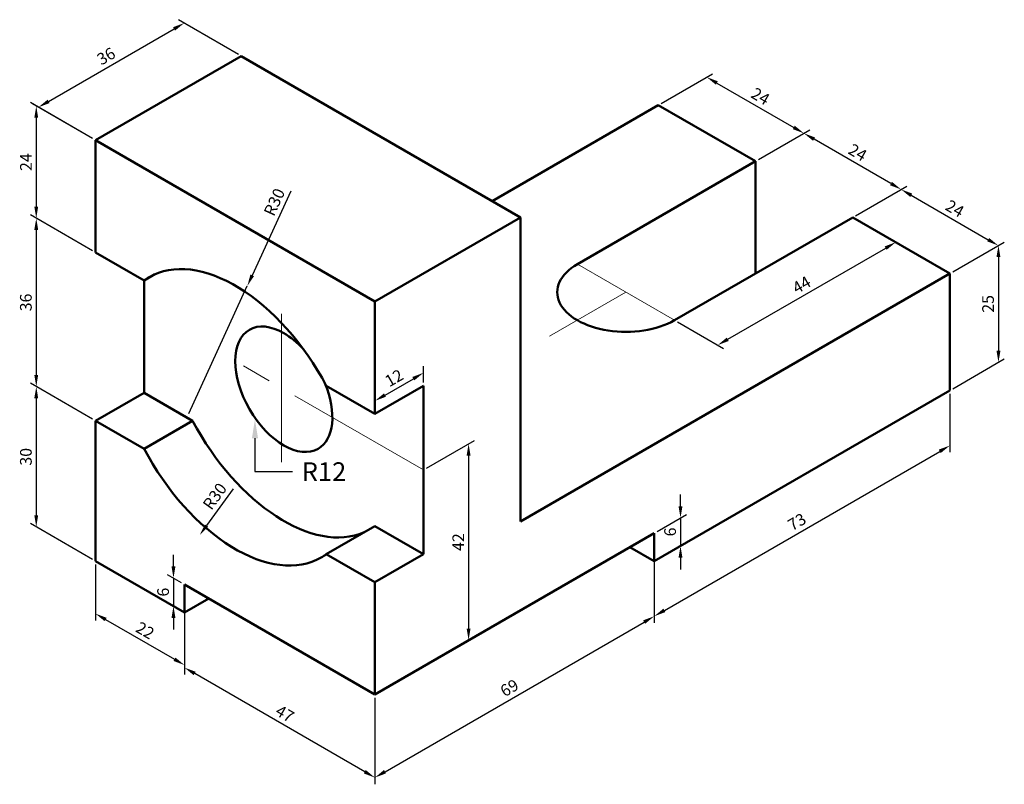
# Model space of a CAD drawing. Units: millimetres. Extents: x 2732 to 2943, y 951 to 1114.
import ezdxf
from ezdxf import colors
from ezdxf.entities.mleader import LeaderData, LeaderLine
from ezdxf.math import Vec2, Vec3

# ---------------------------------------------------------------- set-up
doc = ezdxf.new("R2010")
doc.units = ezdxf.units.MM
doc.linetypes.add('CENTER', pattern=[50.8, 31.75, -6.35, 6.35, -6.35])
for name, color, linetype, lineweight in [('M-CNTR', 1, 'CENTER', 18), ('M-DIMS', 2, 'Continuous', 25), ('M-OUTL', 7, 'Continuous', 50), ('M-TEXT', 3, 'Continuous', 25)]:
    doc.layers.add(name, color=color, linetype=linetype, lineweight=lineweight)
doc.styles.get("Standard").update_dxf_attribs({"font": 'arial.ttf'})
doc.dimstyles.new('ISO-25', dxfattribs={"dimtxt": 2.5, "dimasz": 2.5, "dimexe": 1.25, "dimexo": 0.625, "dimtad": 1, "dimtxsty": 'Standard', "dimcen": 2.5, "dimadec": 0, "dimazin": 0, "dimtfac": 1, "dimtmove": 0, "dimatfit": 3, "dimfxl": 1, "dimarcsym": 0})

# ---------------------------------------------------------------- blocks, each defined once
blk = doc.blocks.new('*D1')
at = {"layer": 'Defpoints', "color": 0, "transparency": 16777216}
for p in [(2910.5, 1072.07), (2941.64, 1066.05), (2931.29, 1060.07)]:
    blk.add_point(p, dxfattribs=at)
at = {"layer": 'M-DIMS', "color": 0, "lineweight": -2, "transparency": 16777216}
for p, q in [((2911.13, 1072.43), (2922.11, 1078.77)), ((2923.02, 1076.8), (2939.48, 1067.3)), ((2931.91, 1060.43), (2942.89, 1066.77))]:
    blk.add_line(p, q, dxfattribs=at)
at = {"layer": 'M-DIMS', "color": 0, "transparency": 16777216}
for points in [[(2923.23, 1077.16), (2922.82, 1076.44), (2920.86, 1078.05)], [(2939.69, 1067.66), (2939.27, 1066.94), (2941.64, 1066.05)]]:
    blk.add_solid(points, dxfattribs=at)
at = {"layer": 'M-DIMS', "color": 0, "transparency": 16777216, "insert": (2932.19, 1073.68), "char_height": 2.5, "attachment_point": 5, "rotation": 330}
blk.add_mtext('24', dxfattribs=at)
blk = doc.blocks.new('*D2')
at = {"layer": 'Defpoints', "color": 0, "transparency": 16777216}
for p in [(2900.07, 1090.05), (2889.72, 1084.07), (2910.5, 1072.07)]:
    blk.add_point(p, dxfattribs=at)
at = {"layer": 'M-DIMS', "color": 0, "lineweight": -2, "transparency": 16777216}
for p, q in [((2890.34, 1084.43), (2901.32, 1090.77)), ((2918.69, 1079.3), (2902.24, 1088.8)), ((2911.13, 1072.43), (2922.11, 1078.77))]:
    blk.add_line(p, q, dxfattribs=at)
at = {"layer": 'M-DIMS', "color": 0, "transparency": 16777216}
for points in [[(2902.45, 1089.16), (2902.03, 1088.44), (2900.07, 1090.05)], [(2918.9, 1079.66), (2918.49, 1078.94), (2920.86, 1078.05)]]:
    blk.add_solid(points, dxfattribs=at)
at = {"layer": 'M-DIMS', "color": 0, "transparency": 16777216, "insert": (2911.41, 1085.68), "char_height": 2.5, "attachment_point": 5, "rotation": 330}
blk.add_mtext('24', dxfattribs=at)
blk = doc.blocks.new('*D3')
at = {"layer": 'Defpoints', "color": 0, "transparency": 16777216}
for p in [(2868.93, 1096.07), (2900.07, 1090.05), (2889.72, 1084.07)]:
    blk.add_point(p, dxfattribs=at)
at = {"layer": 'M-DIMS', "color": 0, "lineweight": -2, "transparency": 16777216}
for p, q in [((2869.56, 1096.43), (2880.54, 1102.77)), ((2881.45, 1100.8), (2897.91, 1091.3)), ((2890.34, 1084.43), (2901.32, 1090.77))]:
    blk.add_line(p, q, dxfattribs=at)
at = {"layer": 'M-DIMS', "color": 0, "transparency": 16777216}
for points in [[(2881.66, 1101.16), (2881.25, 1100.44), (2879.29, 1102.05)], [(2898.12, 1091.66), (2897.7, 1090.94), (2900.07, 1090.05)]]:
    blk.add_solid(points, dxfattribs=at)
at = {"layer": 'M-DIMS', "color": 0, "transparency": 16777216, "insert": (2890.62, 1097.68), "char_height": 2.5, "attachment_point": 5, "rotation": 330}
blk.add_mtext('24', dxfattribs=at)
blk = doc.blocks.new('*D4')
at = {"layer": 'Defpoints', "color": 0, "transparency": 16777216}
for p in [(2931.29, 1060.07), (2941.68, 1041.07), (2931.29, 1035.07)]:
    blk.add_point(p, dxfattribs=at)
at = {"layer": 'M-DIMS', "color": 0, "lineweight": -2, "transparency": 16777216}
for p, q in [((2931.91, 1060.43), (2942.93, 1066.79)), ((2941.68, 1063.57), (2941.68, 1043.57)), ((2931.91, 1035.43), (2942.93, 1041.79))]:
    blk.add_line(p, q, dxfattribs=at)
at = {"layer": 'M-DIMS', "color": 0, "transparency": 16777216}
for points in [[(2941.26, 1063.57), (2942.1, 1063.57), (2941.68, 1066.07)], [(2941.26, 1043.57), (2942.1, 1043.57), (2941.68, 1041.07)]]:
    blk.add_solid(points, dxfattribs=at)
at = {"layer": 'M-DIMS', "color": 0, "transparency": 16777216, "insert": (2939.78, 1053.57), "char_height": 2.5, "attachment_point": 5, "rotation": 90}
blk.add_mtext('25', dxfattribs=at)
blk = doc.blocks.new('*D5')
at = {"layer": 'Defpoints', "color": 0, "transparency": 16777216}
for p in [(2767.53, 1113.62), (2779.73, 1106.57), (2748.55, 1088.57)]:
    blk.add_point(p, dxfattribs=at)
at = {"layer": 'M-DIMS', "color": 0, "lineweight": -2, "transparency": 16777216}
for p, q in [((2779.11, 1106.93), (2766.28, 1114.34)), ((2738.52, 1096.87), (2765.36, 1112.37)), ((2747.93, 1088.93), (2735.1, 1096.34))]:
    blk.add_line(p, q, dxfattribs=at)
at = {"layer": 'M-DIMS', "color": 0, "transparency": 16777216}
for points in [[(2765.16, 1112.73), (2765.57, 1112.01), (2767.53, 1113.62)], [(2738.31, 1097.23), (2738.73, 1096.51), (2736.35, 1095.62)]]:
    blk.add_solid(points, dxfattribs=at)
at = {"layer": 'M-DIMS', "color": 0, "transparency": 16777216, "insert": (2750.99, 1106.26), "char_height": 2.5, "attachment_point": 5, "rotation": 30}
blk.add_mtext('36', dxfattribs=at)
blk = doc.blocks.new('*D6')
at = {"layer": 'Defpoints', "color": 0, "transparency": 16777216}
for p in [(2748.55, 1088.57), (2735.89, 1071.88), (2748.55, 1064.57)]:
    blk.add_point(p, dxfattribs=at)
at = {"layer": 'M-DIMS', "color": 0, "lineweight": -2, "transparency": 16777216}
for p, q in [((2747.93, 1088.93), (2734.64, 1096.61)), ((2735.89, 1093.38), (2735.89, 1074.38)), ((2747.93, 1064.93), (2734.64, 1072.61))]:
    blk.add_line(p, q, dxfattribs=at)
at = {"layer": 'M-DIMS', "color": 0, "transparency": 16777216}
for points in [[(2735.47, 1093.38), (2736.3, 1093.38), (2735.89, 1095.88)], [(2735.47, 1074.38), (2736.3, 1074.38), (2735.89, 1071.88)]]:
    blk.add_solid(points, dxfattribs=at)
at = {"layer": 'M-DIMS', "color": 0, "transparency": 16777216, "insert": (2734.01, 1083.88), "char_height": 2.5, "attachment_point": 5, "rotation": 90}
blk.add_mtext('24', dxfattribs=at)
blk = doc.blocks.new('*D7')
at = {"layer": 'Defpoints', "color": 0, "transparency": 16777216}
for p in [(2748.55, 1064.57), (2735.89, 1035.88), (2748.55, 1028.57)]:
    blk.add_point(p, dxfattribs=at)
at = {"layer": 'M-DIMS', "color": 0, "lineweight": -2, "transparency": 16777216}
for p, q in [((2747.93, 1064.93), (2734.64, 1072.61)), ((2735.89, 1069.38), (2735.89, 1038.38)), ((2747.93, 1028.93), (2734.64, 1036.61))]:
    blk.add_line(p, q, dxfattribs=at)
at = {"layer": 'M-DIMS', "color": 0, "transparency": 16777216}
for points in [[(2735.47, 1069.38), (2736.3, 1069.38), (2735.89, 1071.88)], [(2735.47, 1038.38), (2736.3, 1038.38), (2735.89, 1035.88)]]:
    blk.add_solid(points, dxfattribs=at)
at = {"layer": 'M-DIMS', "color": 0, "transparency": 16777216, "insert": (2733.99, 1053.88), "char_height": 2.5, "attachment_point": 5, "rotation": 90}
blk.add_mtext('36', dxfattribs=at)
blk = doc.blocks.new('*D8')
at = {"layer": 'Defpoints', "color": 0, "transparency": 16777216}
for p in [(2748.55, 1028.57), (2735.89, 1005.88), (2748.55, 998.57)]:
    blk.add_point(p, dxfattribs=at)
at = {"layer": 'M-DIMS', "color": 0, "lineweight": -2, "transparency": 16777216}
for p, q in [((2747.93, 1028.93), (2734.64, 1036.61)), ((2735.89, 1033.38), (2735.89, 1008.38)), ((2747.93, 998.93), (2734.64, 1006.61))]:
    blk.add_line(p, q, dxfattribs=at)
at = {"layer": 'M-DIMS', "color": 0, "transparency": 16777216}
for points in [[(2735.47, 1033.38), (2736.3, 1033.38), (2735.89, 1035.88)], [(2735.47, 1008.38), (2736.3, 1008.38), (2735.89, 1005.88)]]:
    blk.add_solid(points, dxfattribs=at)
at = {"layer": 'M-DIMS', "color": 0, "transparency": 16777216, "insert": (2733.99, 1020.88), "char_height": 2.5, "attachment_point": 5, "rotation": 90}
blk.add_mtext('30', dxfattribs=at)
blk = doc.blocks.new('*D9')
at = {"layer": 'Defpoints', "color": 0, "transparency": 16777216}
for p in [(2748.55, 998.57), (2767.61, 987.57), (2767.61, 976.34)]:
    blk.add_point(p, dxfattribs=at)
at = {"layer": 'M-DIMS', "color": 0, "lineweight": -2, "transparency": 16777216}
for p, q in [((2748.55, 997.85), (2748.55, 985.9)), ((2750.72, 986.09), (2765.44, 977.59)), ((2767.61, 986.85), (2767.61, 974.9))]:
    blk.add_line(p, q, dxfattribs=at)
at = {"layer": 'M-DIMS', "color": 0, "transparency": 16777216}
for points in [[(2750.93, 986.45), (2750.51, 985.73), (2748.55, 987.34)], [(2765.65, 977.95), (2765.23, 977.23), (2767.61, 976.34)]]:
    blk.add_solid(points, dxfattribs=at)
at = {"layer": 'M-DIMS', "color": 0, "transparency": 16777216, "insert": (2759.02, 983.47), "char_height": 2.5, "attachment_point": 5, "rotation": 330}
blk.add_mtext('22', dxfattribs=at)
blk = doc.blocks.new('*D10')
at = {"layer": 'Defpoints', "color": 0, "transparency": 16777216}
for p in [(2767.61, 993.57), (2767.61, 975.79), (2808.31, 970.07)]:
    blk.add_point(p, dxfattribs=at)
at = {"layer": 'M-DIMS', "color": 0, "lineweight": -2, "transparency": 16777216}
for p, q in [((2767.61, 992.85), (2767.61, 974.35)), ((2806.15, 953.54), (2769.77, 974.54)), ((2808.31, 969.35), (2808.31, 950.85))]:
    blk.add_line(p, q, dxfattribs=at)
at = {"layer": 'M-DIMS', "color": 0, "transparency": 16777216}
for points in [[(2769.98, 974.91), (2769.56, 974.18), (2767.61, 975.79)], [(2806.35, 953.91), (2805.94, 953.18), (2808.31, 952.29)]]:
    blk.add_solid(points, dxfattribs=at)
at = {"layer": 'M-DIMS', "color": 0, "transparency": 16777216, "insert": (2788.9, 965.67), "char_height": 2.5, "attachment_point": 5, "rotation": 330}
blk.add_mtext('47', dxfattribs=at)
blk = doc.blocks.new('*D11')
at = {"layer": 'Defpoints', "color": 0, "transparency": 16777216}
for p in [(2868.07, 1004.57), (2868.07, 986.79), (2808.31, 970.07)]:
    blk.add_point(p, dxfattribs=at)
at = {"layer": 'M-DIMS', "color": 0, "lineweight": -2, "transparency": 16777216}
for p, q in [((2868.07, 1003.85), (2868.07, 985.35)), ((2810.48, 953.54), (2865.9, 985.54)), ((2808.31, 969.35), (2808.31, 950.85))]:
    blk.add_line(p, q, dxfattribs=at)
at = {"layer": 'M-DIMS', "color": 0, "transparency": 16777216}
for points in [[(2865.69, 985.91), (2866.11, 985.18), (2868.07, 986.79)], [(2810.27, 953.91), (2810.68, 953.18), (2808.31, 952.29)]]:
    blk.add_solid(points, dxfattribs=at)
at = {"layer": 'M-DIMS', "color": 0, "transparency": 16777216, "insert": (2837.24, 971.19), "char_height": 2.5, "attachment_point": 5, "rotation": 30}
blk.add_mtext('69', dxfattribs=at)
blk = doc.blocks.new('*D12')
at = {"layer": 'Defpoints', "color": 0, "transparency": 16777216}
for p in [(2931.29, 1035.07), (2931.29, 1023.29), (2868.07, 998.57)]:
    blk.add_point(p, dxfattribs=at)
at = {"layer": 'M-DIMS', "color": 0, "lineweight": -2, "transparency": 16777216}
for p, q in [((2931.29, 1034.35), (2931.29, 1021.85)), ((2870.23, 988.04), (2929.12, 1022.04)), ((2868.07, 997.85), (2868.07, 985.35))]:
    blk.add_line(p, q, dxfattribs=at)
at = {"layer": 'M-DIMS', "color": 0, "transparency": 16777216}
for points in [[(2928.91, 1022.41), (2929.33, 1021.68), (2931.29, 1023.29)], [(2870.02, 988.41), (2870.44, 987.68), (2868.07, 986.79)]]:
    blk.add_solid(points, dxfattribs=at)
at = {"layer": 'M-DIMS', "color": 0, "transparency": 16777216, "insert": (2898.73, 1006.69), "char_height": 2.5, "attachment_point": 5, "rotation": 30}
blk.add_mtext('73', dxfattribs=at)
blk = doc.blocks.new('*D13')
at = {"layer": 'Defpoints', "color": 0, "transparency": 16777216}
for p in [(2781.03, 1057.4), (2768.51, 1030.14)]:
    blk.add_point(p, dxfattribs=at)
at = {"layer": 'M-DIMS', "color": 0, "lineweight": -2, "transparency": 16777216}
for p, q in [((2790.35, 1077.69), (2782.07, 1059.67)), ((2768.51, 1030.14), (2781.03, 1057.4))]:
    blk.add_line(p, q, dxfattribs=at)
at = {"layer": 'M-DIMS', "color": 0, "transparency": 16777216}
blk.add_solid([(2781.69, 1059.85), (2782.45, 1059.5), (2781.03, 1057.4)], dxfattribs=at)
at = {"layer": 'M-DIMS', "color": 0, "transparency": 16777216, "insert": (2787.11, 1075.21), "char_height": 2.5, "attachment_point": 5, "rotation": 65.3379}
blk.add_mtext('R30', dxfattribs=at)
blk = doc.blocks.new('*D14')
at = {"layer": 'Defpoints', "color": 0, "transparency": 16777216}
for p in [(2788.35, 1028.51), (2770.85, 1004.14)]:
    blk.add_point(p, dxfattribs=at)
at = {"layer": 'M-DIMS', "color": 0, "lineweight": -2, "transparency": 16777216}
blk.add_line((2777.98, 1014.06), (2772.31, 1006.17), dxfattribs=at)
at = {"layer": 'M-DIMS', "color": 0, "transparency": 16777216}
blk.add_solid([(2771.97, 1006.41), (2772.65, 1005.93), (2770.85, 1004.14)], dxfattribs=at)
at = {"layer": 'M-DIMS', "color": 0, "transparency": 16777216, "insert": (2774.33, 1012.24), "char_height": 2.5, "attachment_point": 5, "rotation": 54.3091}
blk.add_mtext('R30', dxfattribs=at)
blk = doc.blocks.new('*D15')
at = {"layer": 'Defpoints', "color": 0, "transparency": 16777216}
for p in [(2818.7, 1038.83), (2818.7, 1036.07), (2808.31, 1030.07)]:
    blk.add_point(p, dxfattribs=at)
at = {"layer": 'M-DIMS', "color": 0, "lineweight": -2, "transparency": 16777216}
for p, q in [((2818.7, 1036.79), (2818.7, 1040.27)), ((2810.48, 1034.08), (2816.54, 1037.58)), ((2808.31, 1030.79), (2808.31, 1034.27))]:
    blk.add_line(p, q, dxfattribs=at)
at = {"layer": 'M-DIMS', "color": 0, "transparency": 16777216}
for points in [[(2816.33, 1037.94), (2816.75, 1037.22), (2818.7, 1038.83)], [(2810.27, 1034.44), (2810.68, 1033.72), (2808.31, 1032.83)]]:
    blk.add_solid(points, dxfattribs=at)
at = {"layer": 'M-DIMS', "color": 0, "transparency": 16777216, "insert": (2812.57, 1037.46), "char_height": 2.5, "attachment_point": 5, "rotation": 30}
blk.add_mtext('12', dxfattribs=at)
blk = doc.blocks.new('*D16')
at = {"layer": 'Defpoints', "color": 0, "transparency": 16777216}
for p in [(2910.5, 1072.07), (2919.72, 1066.75), (2872.4, 1050.07)]:
    blk.add_point(p, dxfattribs=at)
at = {"layer": 'M-DIMS', "color": 0, "lineweight": -2, "transparency": 16777216}
for p, q in [((2911.13, 1071.71), (2920.97, 1066.03)), ((2883.78, 1046), (2917.56, 1065.5)), ((2873.02, 1049.71), (2882.87, 1044.03))]:
    blk.add_line(p, q, dxfattribs=at)
at = {"layer": 'M-DIMS', "color": 0, "transparency": 16777216}
for points in [[(2917.35, 1065.86), (2917.76, 1065.14), (2919.72, 1066.75)], [(2883.57, 1046.36), (2883.99, 1045.64), (2881.62, 1044.75)]]:
    blk.add_solid(points, dxfattribs=at)
at = {"layer": 'M-DIMS', "color": 0, "transparency": 16777216, "insert": (2899.73, 1057.37), "char_height": 2.5, "attachment_point": 5, "rotation": 30}
blk.add_mtext('44', dxfattribs=at)
blk = doc.blocks.new('*D17')
at = {"layer": 'Defpoints', "color": 0, "transparency": 16777216}
for p in [(2868.07, 1004.57), (2873.68, 1001.81), (2868.07, 998.57)]:
    blk.add_point(p, dxfattribs=at)
at = {"layer": 'M-DIMS', "color": 0, "lineweight": -2, "transparency": 16777216}
for p, q in [((2873.68, 1010.31), (2873.68, 1012.81)), ((2868.69, 1004.93), (2874.93, 1008.53)), ((2873.68, 1007.81), (2873.68, 1001.81)), ((2868.69, 998.93), (2874.93, 1002.53)), ((2873.68, 999.31), (2873.68, 996.81))]:
    blk.add_line(p, q, dxfattribs=at)
at = {"layer": 'M-DIMS', "color": 0, "transparency": 16777216}
for points in [[(2873.26, 1010.31), (2874.09, 1010.31), (2873.68, 1007.81)], [(2873.26, 999.31), (2874.09, 999.31), (2873.68, 1001.81)]]:
    blk.add_solid(points, dxfattribs=at)
at = {"layer": 'M-DIMS', "color": 0, "transparency": 16777216, "insert": (2871.78, 1004.81), "char_height": 2.5, "attachment_point": 5, "rotation": 90}
blk.add_mtext('6', dxfattribs=at)
blk = doc.blocks.new('*D18')
at = {"layer": 'Defpoints', "color": 0, "transparency": 16777216}
for p in [(2767.61, 993.57), (2765.24, 988.94), (2767.61, 987.57)]:
    blk.add_point(p, dxfattribs=at)
at = {"layer": 'M-DIMS', "color": 0, "lineweight": -2, "transparency": 16777216}
for p, q in [((2765.24, 997.44), (2765.24, 999.94)), ((2766.98, 993.93), (2763.99, 995.66)), ((2765.24, 994.94), (2765.24, 988.94)), ((2766.98, 987.93), (2763.99, 989.66)), ((2765.24, 986.44), (2765.24, 983.94))]:
    blk.add_line(p, q, dxfattribs=at)
at = {"layer": 'M-DIMS', "color": 0, "transparency": 16777216}
for points in [[(2764.82, 997.44), (2765.65, 997.44), (2765.24, 994.94)], [(2764.82, 986.44), (2765.65, 986.44), (2765.24, 988.94)]]:
    blk.add_solid(points, dxfattribs=at)
at = {"layer": 'M-DIMS', "color": 0, "transparency": 16777216, "insert": (2763.34, 991.94), "char_height": 2.5, "attachment_point": 5, "rotation": 90}
blk.add_mtext('6', dxfattribs=at)
blk = doc.blocks.new('*D19')
at = {"layer": 'Defpoints', "color": 0, "transparency": 16777216}
for p in [(2818.7, 1018.07), (2828.35, 981.64), (2818.7, 976.07)]:
    blk.add_point(p, dxfattribs=at)
at = {"layer": 'M-DIMS', "color": 0, "lineweight": -2, "transparency": 16777216}
for p, q in [((2819.33, 1018.43), (2829.6, 1024.37)), ((2828.35, 1021.14), (2828.35, 984.14)), ((2819.33, 976.43), (2829.6, 982.37))]:
    blk.add_line(p, q, dxfattribs=at)
at = {"layer": 'M-DIMS', "color": 0, "transparency": 16777216}
for points in [[(2827.94, 1021.14), (2828.77, 1021.14), (2828.35, 1023.64)], [(2827.94, 984.14), (2828.77, 984.14), (2828.35, 981.64)]]:
    blk.add_solid(points, dxfattribs=at)
at = {"layer": 'M-DIMS', "color": 0, "transparency": 16777216, "insert": (2826.47, 1002.64), "char_height": 2.5, "attachment_point": 5, "rotation": 90}
blk.add_mtext('42', dxfattribs=at)

msp = doc.modelspace()

# ---------------------------------------------------------------- linework, layer by layer
at = {"layer": 'M-CNTR'}
for p, q in [((2872.396, 1050.072), (2851.612, 1062.072)), ((2788.354, 1019.7), (2788.354, 1057.468)), ((2862.004, 1056.072), (2845.689, 1046.652)), ((2818.703, 1018.072), (2776.499, 1042.438)), ((2868.066, 998.572), (2862.87, 1001.572))]:
    msp.add_line(p, q, dxfattribs=at)
at = {"layer": 'M-OUTL'}
for p, q in [((2748.555, 1088.572), (2779.732, 1106.572)), ((2779.732, 1106.572), (2839.487, 1072.072)), ((2868.932, 1096.072), (2833.425, 1075.572)), ((2889.717, 1084.072), (2868.932, 1096.072)), ((2808.311, 1054.072), (2748.555, 1088.572)), ((2748.555, 1088.572), (2748.555, 1064.572)), ((2851.612, 1062.072), (2889.717, 1084.072)), ((2889.717, 1060.072), (2889.717, 1084.072)), ((2839.487, 1072.072), (2808.311, 1054.072)), ((2839.487, 1072.072), (2839.487, 1007.072)), ((2910.502, 1072.072), (2872.396, 1050.072)), ((2931.286, 1060.072), (2910.502, 1072.072)), ((2748.555, 1064.572), (2758.947, 1058.572)), ((2758.948, 1058.572), (2761.249, 1059.9)), ((2931.286, 1060.072), (2839.487, 1007.072)), ((2931.286, 1035.072), (2931.286, 1060.072)), ((2758.947, 1058.572), (2758.947, 1034.572)), ((2808.311, 1030.072), (2808.311, 1054.072)), ((2758.947, 1034.572), (2748.555, 1028.572)), ((2769.339, 1028.572), (2758.947, 1034.572)), ((2808.311, 1030.072), (2797.918, 1036.072)), ((2818.703, 1036.072), (2808.311, 1030.072)), ((2818.703, 1000.072), (2818.703, 1036.072)), ((2868.066, 998.572), (2931.286, 1035.072)), ((2748.555, 998.572), (2748.555, 1028.572)), ((2748.555, 1028.572), (2758.947, 1022.572)), ((2758.947, 1022.572), (2769.339, 1028.572)), ((2818.703, 1000.072), (2818.703, 1018.072)), ((2808.311, 1006.072), (2797.918, 1000.072)), ((2818.703, 1000.072), (2808.311, 1006.072)), ((2808.311, 970.072), (2868.066, 1004.572)), ((2868.066, 1004.572), (2868.066, 998.572)), ((2868.067, 998.572), (2862.871, 1001.572)), ((2767.607, 987.572), (2748.555, 998.572)), ((2797.918, 1000.072), (2808.311, 994.072)), ((2808.311, 994.072), (2818.703, 1000.072)), ((2808.311, 970.072), (2808.311, 994.072)), ((2808.311, 970.072), (2767.607, 993.572)), ((2767.607, 993.572), (2767.607, 987.572)), ((2767.607, 987.572), (2772.804, 990.572))]:
    msp.add_line(p, q, dxfattribs=at)
for centre, major_axis, start_param, end_param in [((2778.433, 1027.479), (18.371, -31.82), 1.5081225, 3.1415927), ((2862.004, 1056.072), (-14.697, 0), 5.4977871, 8.6393798), ((2778.433, 1027.479), (18.371, -31.82), 3.1415927, 3.2042665), ((2788.825, 1035.322), (7.348, -12.728), 2.3561945, 3.1415927), ((2788.825, 1035.322), (7.348, -12.728), 3.1415927, 6.2831853), ((2788.825, 1035.322), (7.348, -12.728), 1.9395001, 2.3561945), ((2788.825, 1035.322), (7.348, -12.728), 0, 1.3444632), ((2788.825, 1037.165), (18.371, -31.82), 4.6497151, 6.2205114), ((2778.433, 1031.165), (18.371, -31.82), 4.6497151, 6.2831853), ((2778.433, 1031.165), (18.371, -31.82), 0, 0.0626739)]:
    msp.add_ellipse(centre, major_axis=major_axis, ratio=0.5773503, start_param=start_param, end_param=end_param, dxfattribs=at)

# ---------------------------------------------------------------- dimensions: what is measured, and where the dimension line sits
at = {"layer": 'M-DIMS'}
for p1, p2, distance, picture, middle in [((2748.555, 1088.572), (2779.732, 1106.572), 12.203, '*D5', (2750.989, 1106.265)), ((2868.932, 1096.072), (2889.717, 1084.072), 10.357, '*D3', (2890.622, 1097.68)), ((2748.555, 1088.572), (2748.555, 1064.572), -12.667, '*D6', (2734.008, 1083.885)), ((2910.502, 1072.072), (2889.717, 1084.072), -10.357, '*D2', (2911.406, 1085.68)), ((2910.502, 1072.072), (2931.286, 1060.072), 10.357, '*D1', (2932.191, 1073.68)), ((2748.555, 1064.572), (2748.555, 1028.572), -12.667, '*D7', (2733.986, 1053.885)), ((2872.396, 1050.072), (2910.502, 1072.072), -9.22, '*D16', (2899.731, 1057.373)), ((2931.286, 1060.072), (2931.286, 1035.072), 10.394, '*D4', (2939.779, 1053.573)), ((2808.311, 1030.072), (2818.703, 1036.072), 2.388, '*D15', (2812.567, 1037.457)), ((2748.555, 1028.572), (2748.555, 998.572), -12.667, '*D8', (2733.986, 1020.885)), ((2868.066, 998.572), (2931.286, 1035.072), -10.199, '*D12', (2898.725, 1006.692)), ((2818.703, 1018.072), (2818.703, 976.072), 9.65, '*D19', (2826.473, 1002.643)), ((2868.066, 1004.572), (2868.066, 998.572), 5.611, '*D17', (2871.776, 1004.811)), ((2808.311, 970.072), (2868.066, 1004.572), -15.396, '*D11', (2837.238, 971.191)), ((2748.555, 998.572), (2767.607, 987.572), -9.728, '*D9', (2759.021, 983.467)), ((2767.607, 993.572), (2767.607, 987.572), -2.37, '*D18', (2763.336, 991.94)), ((2808.311, 970.072), (2767.607, 993.572), 15.396, '*D10', (2788.896, 965.668))]:
    dim = msp.add_aligned_dim(p1=p1, p2=p2, distance=distance, dimstyle='ISO-25', override={"dimclrd": 0, "dimclre": 0, "dimclrt": 0}, dxfattribs=at)
    dim.commit()
    dim.dimension.update_dxf_attribs({"geometry": picture, "text_midpoint": middle})
for center, mpoint, picture, middle in [((2768.511, 1030.137), (2781.029, 1057.401), '*D13', (2788.84, 1074.412)), ((2788.354, 1028.506), (2770.852, 1004.141), '*D14', (2775.874, 1011.132))]:
    dim = msp.add_radius_dim(center=center, mpoint=mpoint, dimstyle='ISO-25', override={"dimclrd": 0, "dimclre": 0, "dimclrt": 0}, dxfattribs=at)
    dim.commit()
    dim.dimension.update_dxf_attribs({"geometry": picture, "text_midpoint": middle, "dimtype": 164})

# ---------------------------------------------------------------- leaders
at = {"layer": 'M-TEXT'}
ml = msp.add_multileader_mtext('Standard', dxfattribs=at)
ml.set_content('R12', color=256)
ml.set_leader_properties()
ml.build(insert=Vec2(0, 0))
ctx = ml.context
ctx.base_point, ctx.plane_origin = Vec3(2790.664, 1017.703), Vec3(2782.664, 1028.838)
notes = []
notes.append((ctx, [(0, (1, 1, 0), (2782.664, 1017.703), (1, 0), 8, [(0, [(2782.664, 1028.838)], 0, [])])]))
ctx.mtext.insert, ctx.mtext.flow_direction = Vec3(2792.664, 1019.703), 5
for ctx, leaders in notes:
    for number, flags, end, landing, length, lines in leaders:
        leader = LeaderData()
        leader.index, (leader.has_last_leader_line, leader.has_dogleg_vector, leader.attachment_direction) = number, flags
        leader.last_leader_point, leader.dogleg_vector, leader.dogleg_length = Vec3(end), Vec3(landing), length
        for number, points, colour, breaks in lines:
            line = LeaderLine()
            line.index, line.vertices, line.color, line.breaks = number, Vec3.list(points), colors.encode_raw_color(colour), breaks
            leader.lines.append(line)
        ctx.leaders.append(leader)

doc.saveas('drawing.dxf')
